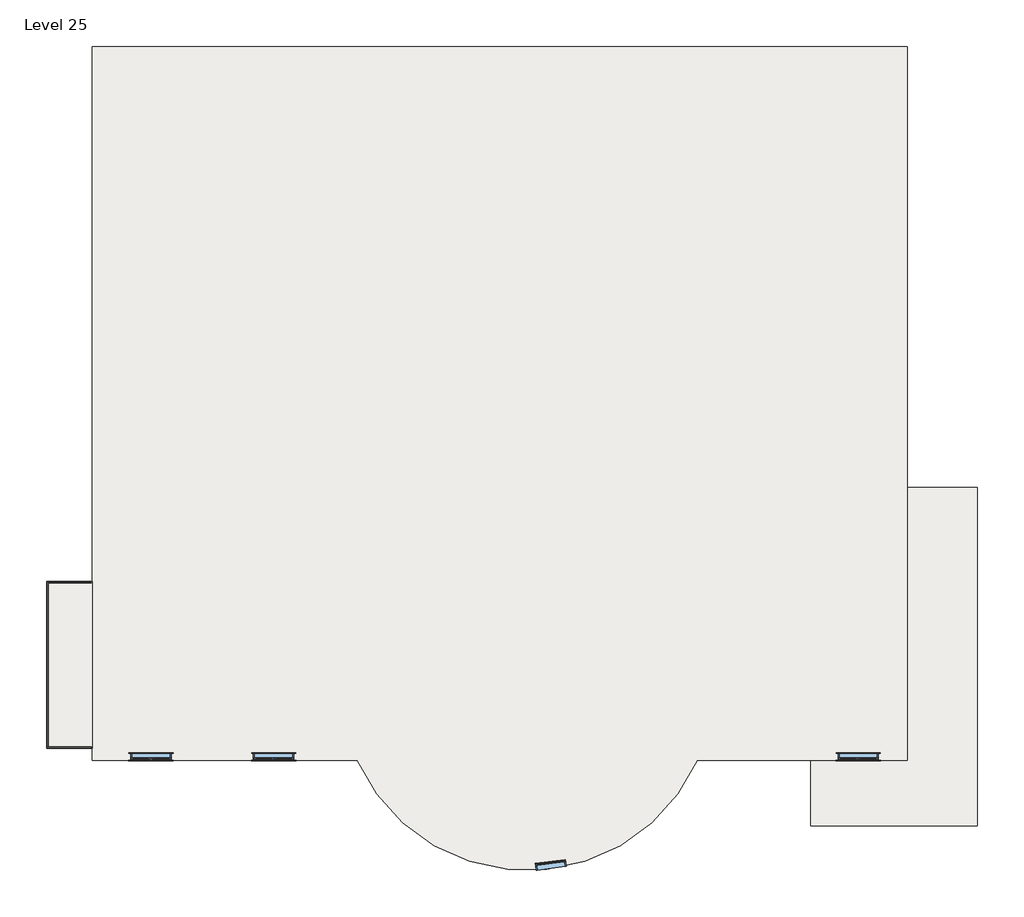
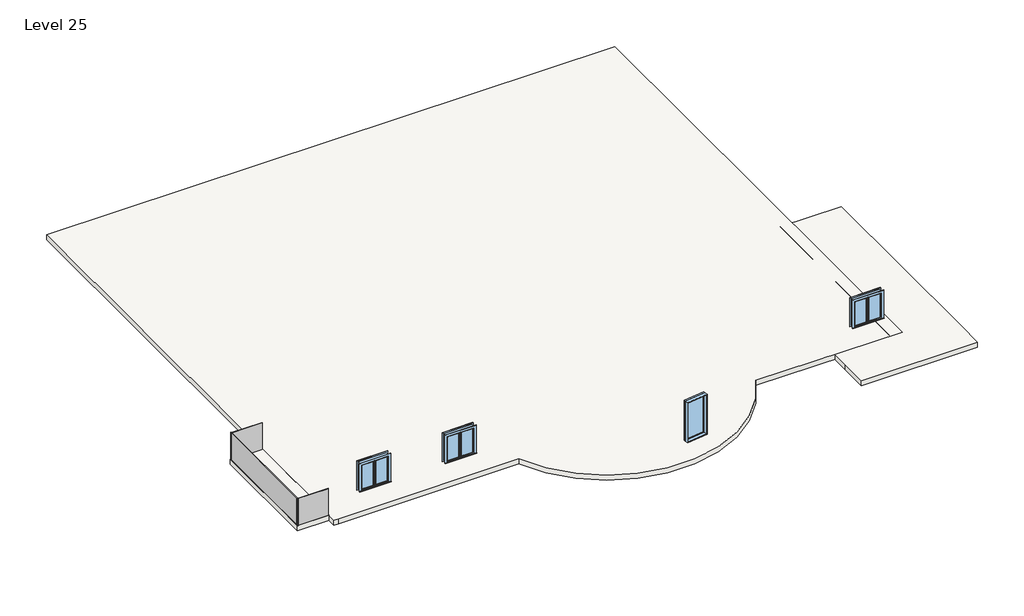
# One storey: 4 windows, 3 plates, 3 slabs.
"""IFC4 building model written with IfcOpenShell, lengths in millimetres."""

from ifc_helpers import new_model, si_unit, point, frame, frame_2d, origin, place, context, project, spatial, polyline, circle_curve, trimmed, segment, composite_curve, outline, extrude, transform, mapped, element, save
from components import system_panel_glazed_7d767388, system_panel_glazed_c55d8a5b, system_panel_glazed_9f710733, window_0862ab64, window_9a779fa2

model = new_model("IFC4")

# Units and contexts
model_context = context("Model", 3, world=origin())
ifc_project = project(units=[si_unit("LENGTHUNIT", "METRE", prefix="MILLI")], contexts=[model_context])

# Site, building, storey
site = spatial("IfcSite", under=ifc_project)
building = spatial("IfcBuilding", under=site)
storey = spatial("IfcBuildingStorey", under=building, Name="Level 25", Elevation=39319.2)

# Plates
placement = place(None, origin())
system_panel_glazed_shape = system_panel_glazed_7d767388(model_context)
element("IfcPlate", 1, ObjectType="System Panel : Glazed", at=placement, inside=storey, context=model_context, shape_type="MappedRepresentation", body=[
    mapped(system_panel_glazed_shape, transform((-17306.4505427, -8690.0239591, 39319.2), x_axis=(-1.0, 0.0, 0.0), y_axis=(0.0, -1.0, 0.0), z_axis=(0.0, 0.0, 1.0))),
])
system_panel_glazed_2_shape = system_panel_glazed_c55d8a5b(model_context)
element("IfcPlate", 2, ObjectType="System Panel : Glazed", at=placement, inside=storey, context=model_context, shape_type="MappedRepresentation", body=[
    mapped(system_panel_glazed_2_shape, transform((-17979.5505427, -11204.6239591, 39319.2), x_axis=(0.0, -1.0, 0.0), y_axis=(1.0, 0.0, 0.0), z_axis=(0.0, 0.0, 1.0))),
])
system_panel_glazed_3_shape = system_panel_glazed_9f710733(model_context)
element("IfcPlate", 3, ObjectType="System Panel : Glazed", at=placement, inside=storey, context=model_context, shape_type="MappedRepresentation", body=[
    mapped(system_panel_glazed_3_shape, transform((-17302.8277899, -13719.2239591, 39319.2), x_axis=(1.0, 0.0, 0.0), y_axis=(0.0, 1.0, 0.0), z_axis=(0.0, 0.0, 1.0))),
])

# Slabs
element("IfcSlab", 4, ObjectType="9\"", at=placement, inside=storey, context=model_context, shape_type="SweptSolid", body=[
    extrude(outline(composite_curve([segment(polyline([(-16607.9505427, 7461.1191779), (7979.2494573, 7461.1191779), (7979.2494573, -14078.0808221), (1652.8739931, -14078.0808221)]), True, "CONTINUOUS"), segment(trimmed(circle_curve(frame_2d((-3476.1505427, -11788.3650223)), 5616.9111737), [point((1652.8739931, -14078.0808221))], [point((-8605.1750786, -14078.0808221))], False, "CARTESIAN"), True, "CONTINUOUS"), segment(polyline([(-8605.1750786, -14078.0808221), (-16404.7505427, -14078.0808221), (-16607.9505427, -14078.0808221), (-16607.9505427, 7461.1191779)]), True, "CONTINUOUS")], self_intersect=False)), frame((0.0, 0.0, 39090.6), z_axis=(0.0, 0.0, 1.0), x_axis=(1.0, 0.0, 0.0)), (0.0, 0.0, 1.0), 228.6),
])
element("IfcSlab", 5, ObjectType="9\"", at=placement, inside=storey, context=model_context, shape_type="SweptSolid", body=[
    extrude(outline(polyline([(-17978.526008, -8690.0239591), (-16606.926008, -8690.0239591), (-16606.926008, -13719.2239591), (-17978.526008, -13719.2239591), (-17978.526008, -8690.0239591)])), frame((0.0, 0.0, 39090.6), z_axis=(0.0, 0.0, 1.0), x_axis=(1.0, 0.0, 0.0)), (0.0, 0.0, 1.0), 228.6),
])
element("IfcSlab", 6, ObjectType="9\"", at=placement, inside=storey, context=model_context, shape_type="SweptSolid", body=[
    extrude(outline(polyline([(5071.4396352, -14840.0808221), (5071.4396352, -14078.0808221), (7255.8396352, -14078.0808221), (7459.0396352, -14078.0808221), (7459.0396352, -5848.4808221), (10100.6396352, -5848.4808221), (10100.6396352, -14840.0808221), (10100.6396352, -16059.2808221), (5071.4396352, -16059.2808221), (5071.4396352, -14840.0808221)])), frame((0.0, 0.0, 39090.6), z_axis=(0.0, 0.0, 1.0), x_axis=(1.0, 0.0, 0.0)), (0.0, 0.0, 1.0), 228.6),
])

# Windows
window_shape = window_0862ab64(model_context)
element("IfcWindow", 7, ObjectType="Casement Dbl with Trim : 48\" x 48\"", at=placement, inside=storey, context=model_context, shape_type="MappedRepresentation", body=[
    mapped(window_shape, transform((-14829.9505427, -13957.4308221, 39319.2), x_axis=(-1.0, 0.0, 0.0), y_axis=(0.0, -1.0, 0.0), z_axis=(0.0, 0.0, 1.0))),
])
element("IfcWindow", 8, ObjectType="Casement Dbl with Trim : 48\" x 48\"", at=placement, inside=storey, context=model_context, shape_type="MappedRepresentation", body=[
    mapped(window_shape, transform((-11129.6382271, -13957.4308221, 39319.2), x_axis=(-1.0, 0.0, 0.0), y_axis=(0.0, -1.0, 0.0), z_axis=(0.0, 0.0, 1.0))),
])
element("IfcWindow", 9, ObjectType="Casement Dbl with Trim : 48\" x 48\"", at=placement, inside=storey, context=model_context, shape_type="MappedRepresentation", body=[
    mapped(window_shape, transform((6506.0494573, -13957.4308221, 39319.2), x_axis=(-1.0, 0.0, 0.0), y_axis=(0.0, -1.0, 0.0), z_axis=(0.0, 0.0, 1.0))),
])
window_2_shape = window_9a779fa2(model_context)
element("IfcWindow", 10, ObjectType="Fixed : 36\" x 72\"", at=placement, inside=storey, context=model_context, shape_type="MappedRepresentation", body=[
    mapped(window_2_shape, transform((-2733.9537497, -17234.1240216, 39877.4775112), x_axis=(0.9917523902379195, 0.12816862508965818, 0.0), y_axis=(-0.12816862508965818, 0.9917523902379195, 0.0), z_axis=(0.0, 0.0, 1.0))),
])

save(model, "model.ifc")

# Revit data of these elements
# Type "System Panel : Glazed"
#   Construction Type Id = "GSP4R"
#   Analytic Construction = "1/8 in Pilkington single glazing"
#   Visual Light Transmittance = 0.9
#   Solar Heat Gain Coefficient = 0.86
#   Heat Transfer Coefficient (U) = 1.18115 BTU/(h·ft²·°F)
# Type "9\""
#   Assembly Code = "B1010"
#   Function = 0
#   Layers, outside or top first: 0' - 9" no material (function 1)
# Type "Casement Dbl with Trim : 48\" x 48\""
#   Type Mark = "10"
#   Construction Type Id = "GSP4R"
#   Assembly Code = "B2020100"
#   Analytic Construction = "1/8 in Pilkington single glazing"
#   Visual Light Transmittance = 0.9
#   Solar Heat Gain Coefficient = 0.78
#   Heat Transfer Coefficient (U) = 0.6496 BTU/(h·ft²·°F)
#   Height = 4' - 0"
#   Default Sill Height = 3' - 0"
#   Trim Projection - Ext. = 0' - 0 1/2"
#   Trim Projection - Int. = 0' - 0 3/4"
#   Trim Width - Exterior = 0' - 3 1/2"
#   Trim Width - Interior = 0' - 3 1/2"
#   Width = 4' - 0"
#   Window Inset = 0' - 0 3/4"
#   Define Thermal Properties by = 1
#   Glass Pane Material = Glass
#   Sash Material = Sash
#   Trim Exterior Material = Trim
#   Trim Interior Material = Trim
#   Wall Closure = (empty or 0)
# Type "Fixed : 36\" x 72\""
#   Type Mark = "9"
#   Construction Type Id = "GSP4R"
#   Assembly Code = "B2020100"
#   Analytic Construction = "1/8 in Pilkington single glazing"
#   Visual Light Transmittance = 0.9
#   Solar Heat Gain Coefficient = 0.78
#   Heat Transfer Coefficient (U) = 0.6496 BTU/(h·ft²·°F)
#   Height = 6' - 0"
#   Default Sill Height = 1' - 0"
#   Width = 3' - 0"
#   Window Inset = 0' - 0 3/4"
#   Define Thermal Properties by = 1
#   Glass Pane Material = Glass
#   Sash Material = Sash
#   Wall Closure = (empty or 0)
# Elements 1, 2, 3 (IfcPlate, "System Panel : Glazed")
#   Phase Created = New Construction
#   Materials on its faces: "Glass"
# Element 4 (IfcSlab, "9\"")
#   built-in parameter 1001955 = 1.5708 (stored number, unit not read)
#   Height Offset From Level = 0' - 0"
#   Phase Created = New Construction
#   Materials on its faces: "Default Floor"
# Element 5 (IfcSlab, "9\"")
#   built-in parameter 1001955 = 3.14159 (stored number, unit not read)
#   Height Offset From Level = 0' - 0"
#   Phase Created = New Construction
#   Materials on its faces: "Default Floor"
# Element 6 (IfcSlab, "9\"")
#   built-in parameter 1001955 = -1.5708 (stored number, unit not read)
#   Height Offset From Level = 0' - 0"
#   Phase Created = New Construction
#   Materials on its faces: "Default Floor"
# Element 7 (IfcWindow, "Casement Dbl with Trim : 48\" x 48\"")
#   Mark = "23"
#   Phase Created = New Construction
#   Materials on its faces: "Sash", "Trim", "Glass"
# Element 8 (IfcWindow, "Casement Dbl with Trim : 48\" x 48\"")
#   Mark = "24"
#   Phase Created = New Construction
#   Materials on its faces: "Sash", "Trim", "Glass"
# Element 9 (IfcWindow, "Casement Dbl with Trim : 48\" x 48\"")
#   Mark = "49"
#   Phase Created = New Construction
#   Materials on its faces: "Sash", "Trim", "Glass"
# Element 10 (IfcWindow, "Fixed : 36\" x 72\"")
#   Mark = "4"
#   Phase Created = New Construction
#   Materials on its faces: "Sash", "Glass"
# Materials
#   "Glass": class "Glass", colour RGB 0 128 192, transparency 0.75, Description = "Soda Lime Glass", Cost = 0
#   "Sash": class "Wood", colour RGB 224 178 126, transparency 0
#   "Trim": class "Wood", colour RGB 224 178 126, transparency 0
#   "Default Floor": colour RGB 128 128 128, transparency 0
